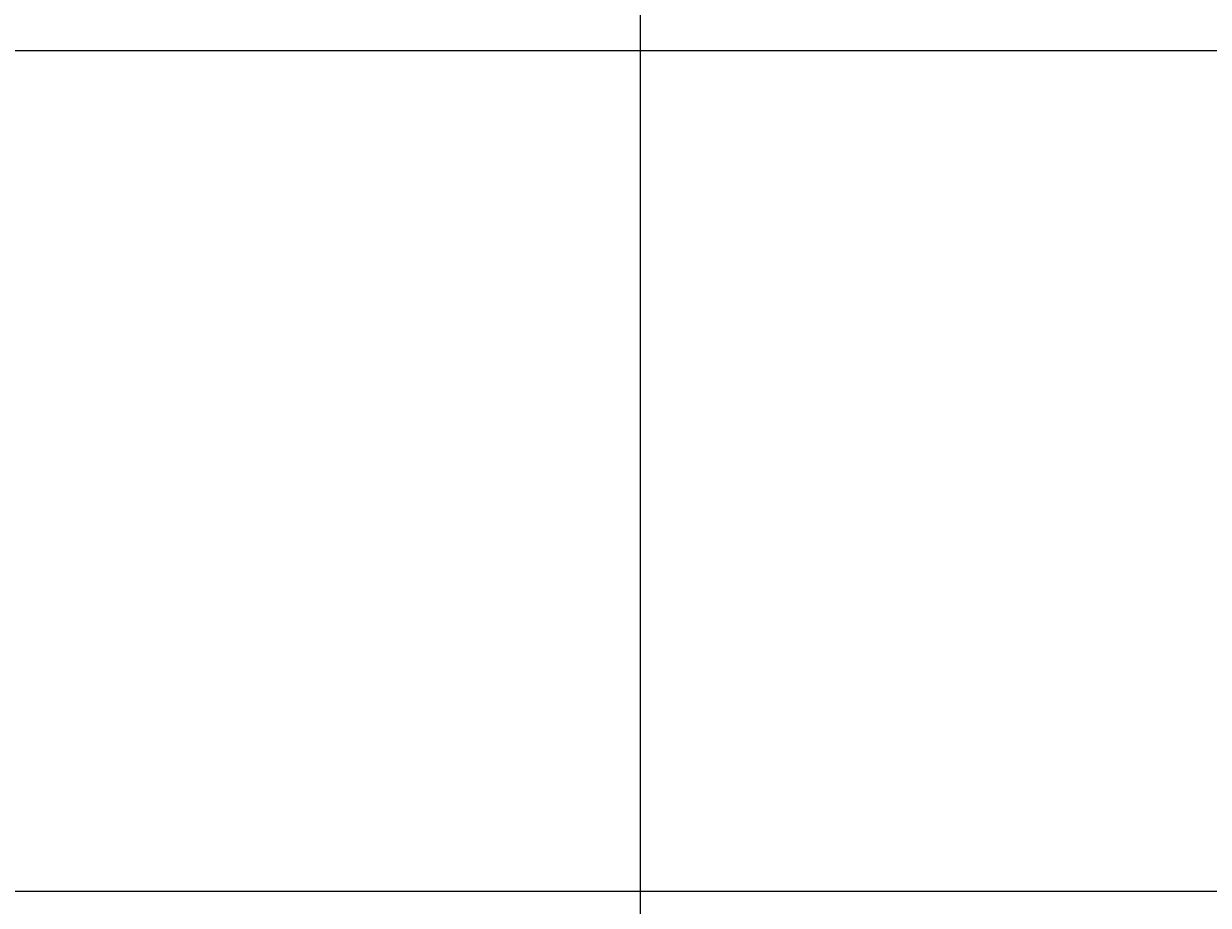
# Model space of a CAD drawing. Units: inches. Extents: x 35362 to 73946, y 43607 to 67532.
# Tile 92 of 134: x 49711 to 50119, y 48965 to 49269. Entities that reach past the tile are written whole.
import ezdxf

# ---------------------------------------------------------------- set-up
doc = ezdxf.new("R2010")
doc.units = ezdxf.units.IN
doc.header["$MEASUREMENT"] = 0
doc.layers.add('A-ANNO-DIMS', color=2, linetype='Continuous', lineweight=18)
doc.styles.get("Standard").update_dxf_attribs({"font": 'arial.ttf'})
doc.dimstyles.get("Standard").update_dxf_attribs({"dimtxt": 0.18, "dimasz": 0.18, "dimexe": 0.18, "dimexo": 0.0625, "dimgap": 0.09, "dimtad": 0, "dimtih": 1, "dimtoh": 1, "dimdec": 4, "dimzin": 0, "dimdsep": 46, "dimtxsty": 'Standard', "dimcen": 0.09, "dimadec": 0, "dimazin": 0, "dimtfac": 1, "dimtdec": 4, "dimtofl": 0, "dimtmove": 0, "dimatfit": 3, "dimfxl": 1, "dimtolj": 1, "dimtzin": 0, "dimarcsym": 0})

# ---------------------------------------------------------------- blocks, each defined once
blk = doc.blocks.new('*D11')
at = {"layer": 'A-ANNO-DIMS', "color": 0, "lineweight": -2, "transparency": 16777216}
for p, q in [((47978.66, 56028.77), (47978.66, 43606.68)), ((53109.76, 56028.77), (53109.76, 43606.68)), ((47978.84, 43606.86), (50543.87, 43606.86)), ((53109.58, 43606.86), (50544.55, 43606.86))]:
    blk.add_line(p, q, dxfattribs=at)
at = {"layer": 'A-ANNO-DIMS', "color": 0, "transparency": 16777216}
for points in [[(47978.84, 43606.89), (47978.84, 43606.83), (47978.66, 43606.86)], [(53109.58, 43606.89), (53109.58, 43606.83), (53109.76, 43606.86)]]:
    blk.add_solid(points, dxfattribs=at)
at = {"layer": 'Defpoints', "color": 0, "transparency": 16777216}
for p in [(47978.66, 56028.84), (53109.76, 56028.84), (53109.76, 43606.86)]:
    blk.add_point(p, dxfattribs=at)
at = {"layer": 'A-ANNO-DIMS', "color": 0, "transparency": 16777216, "insert": (50544.21, 43606.86), "char_height": 0.18, "attachment_point": 5}
blk.add_mtext('\\A1;5131', dxfattribs=at)
blk = doc.blocks.new('*D13')
at = {"layer": 'A-ANNO-DIMS', "color": 0, "lineweight": -2, "transparency": 16777216}
for p, q in [((48373.49, 51694.02), (48373.49, 43606.68)), ((51029.04, 51694.02), (51029.04, 43606.68)), ((48373.67, 43606.86), (49700.8, 43606.86)), ((51028.86, 43606.86), (49701.73, 43606.86))]:
    blk.add_line(p, q, dxfattribs=at)
at = {"layer": 'A-ANNO-DIMS', "color": 0, "transparency": 16777216}
for points in [[(48373.67, 43606.89), (48373.67, 43606.83), (48373.49, 43606.86)], [(51028.86, 43606.89), (51028.86, 43606.83), (51029.04, 43606.86)]]:
    blk.add_solid(points, dxfattribs=at)
at = {"layer": 'Defpoints', "color": 0, "transparency": 16777216}
for p in [(48373.49, 51694.09), (51029.04, 51694.09), (51029.04, 43606.86)]:
    blk.add_point(p, dxfattribs=at)
at = {"layer": 'A-ANNO-DIMS', "color": 0, "transparency": 16777216, "insert": (49701.27, 43606.86), "char_height": 0.18, "attachment_point": 5}
blk.add_mtext('\\A1;2655.6', dxfattribs=at)
blk = doc.blocks.new('*D17')
at = {"layer": 'A-ANNO-DIMS', "color": 0, "lineweight": -2, "transparency": 16777216}
for p, q in [((49923.31, 61293.22), (49923.31, 43606.68)), ((51913.93, 61293.22), (51913.93, 43606.68)), ((49923.49, 43606.86), (50918.16, 43606.86)), ((51913.75, 43606.86), (50919.07, 43606.86))]:
    blk.add_line(p, q, dxfattribs=at)
at = {"layer": 'A-ANNO-DIMS', "color": 0, "transparency": 16777216}
for points in [[(49923.49, 43606.89), (49923.49, 43606.83), (49923.31, 43606.86)], [(51913.75, 43606.89), (51913.75, 43606.83), (51913.93, 43606.86)]]:
    blk.add_solid(points, dxfattribs=at)
at = {"layer": 'Defpoints', "color": 0, "transparency": 16777216}
for p in [(49923.31, 61293.29), (51913.93, 61293.29), (51913.93, 43606.86)]:
    blk.add_point(p, dxfattribs=at)
at = {"layer": 'A-ANNO-DIMS', "color": 0, "transparency": 16777216, "insert": (50918.62, 43606.86), "char_height": 0.18, "attachment_point": 5}
blk.add_mtext('\\A1;1990.6', dxfattribs=at)
blk = doc.blocks.new('*D67')
at = {"layer": 'A-ANNO-DIMS', "color": 0, "lineweight": -2, "transparency": 16777216}
for p, q in [((56873.54, 53351.53), (35361.77, 53351.53)), ((35361.95, 53351.35), (35361.95, 49400.89)), ((35361.95, 45450.07), (35361.95, 49400.53)), ((53793.58, 45449.89), (35361.77, 45449.89))]:
    blk.add_line(p, q, dxfattribs=at)
at = {"layer": 'A-ANNO-DIMS', "color": 0, "transparency": 16777216}
for points in [[(35361.92, 53351.35), (35361.98, 53351.35), (35361.95, 53351.53)], [(35361.92, 45450.07), (35361.98, 45450.07), (35361.95, 45449.89)]]:
    blk.add_solid(points, dxfattribs=at)
at = {"layer": 'Defpoints', "color": 0, "transparency": 16777216}
for p in [(35361.95, 53351.53), (56873.6, 53351.53), (53793.64, 45449.89)]:
    blk.add_point(p, dxfattribs=at)
at = {"layer": 'A-ANNO-DIMS', "color": 0, "transparency": 16777216, "insert": (35361.95, 49400.71), "char_height": 0.18, "attachment_point": 5}
blk.add_mtext('\\A1;7901.6', dxfattribs=at)
blk = doc.blocks.new('*D84')
at = {"layer": 'A-ANNO-DIMS', "color": 0, "lineweight": -2, "transparency": 16777216}
for p, q in [((55540.23, 49259.94), (35361.77, 49259.94)), ((35361.95, 49259.76), (35361.95, 49115.14)), ((35361.95, 48970.16), (35361.95, 49114.78)), ((55540.23, 48969.98), (35361.77, 48969.98))]:
    blk.add_line(p, q, dxfattribs=at)
at = {"layer": 'A-ANNO-DIMS', "color": 0, "transparency": 16777216}
for points in [[(35361.92, 49259.76), (35361.98, 49259.76), (35361.95, 49259.94)], [(35361.92, 48970.16), (35361.98, 48970.16), (35361.95, 48969.98)]]:
    blk.add_solid(points, dxfattribs=at)
at = {"layer": 'Defpoints', "color": 0, "transparency": 16777216}
for p in [(35361.95, 49259.94), (55540.3, 49259.94), (55540.3, 48969.98)]:
    blk.add_point(p, dxfattribs=at)
at = {"layer": 'A-ANNO-DIMS', "color": 0, "transparency": 16777216, "insert": (35361.95, 49114.96), "char_height": 0.18, "attachment_point": 5}
blk.add_mtext('\\A1;289.96', dxfattribs=at)
blk = doc.blocks.new('*D86')
at = {"layer": 'A-ANNO-DIMS', "color": 0, "lineweight": -2, "transparency": 16777216}
for p, q in [((51285.53, 49320.08), (35361.77, 49320.08)), ((35361.95, 49319.9), (35361.95, 49120.26)), ((35361.95, 48920.26), (35361.95, 49119.9)), ((51285.53, 48920.08), (35361.77, 48920.08))]:
    blk.add_line(p, q, dxfattribs=at)
at = {"layer": 'A-ANNO-DIMS', "color": 0, "transparency": 16777216}
for points in [[(35361.92, 49319.9), (35361.98, 49319.9), (35361.95, 49320.08)], [(35361.92, 48920.26), (35361.98, 48920.26), (35361.95, 48920.08)]]:
    blk.add_solid(points, dxfattribs=at)
at = {"layer": 'Defpoints', "color": 0, "transparency": 16777216}
for p in [(35361.95, 49320.08), (51285.59, 49320.08), (51285.59, 48920.08)]:
    blk.add_point(p, dxfattribs=at)
at = {"layer": 'A-ANNO-DIMS', "color": 0, "transparency": 16777216, "insert": (35361.95, 49120.08), "char_height": 0.18, "attachment_point": 5}
blk.add_mtext('\\A1;400.0', dxfattribs=at)

msp = doc.modelspace()

# ---------------------------------------------------------------- dimensions: what is measured, and where the dimension line sits
at = {"layer": 'A-ANNO-DIMS'}
for base, p1, p2, override, picture, middle in [((51913.931, 43606.859), (49923.307, 61293.286), (51913.931, 61293.286), {"dimdec": 1, "dimlfac": 1, "dimrnd": 0, "dimzin": 0, "dimdsep": 46, "dimlunit": 2}, '*D17', (50918.619, 43606.859)), ((53109.76, 43606.859), (47978.665, 56028.836), (53109.76, 56028.836), {"dimdec": 0, "dimlfac": 1, "dimrnd": 0, "dimzin": 0, "dimdsep": 46, "dimlunit": 2}, '*D11', (50544.212, 43606.859)), ((51029.043, 43606.859), (48373.492, 51694.087), (51029.043, 51694.087), {"dimdec": 1, "dimlfac": 1, "dimrnd": 0, "dimzin": 0, "dimdsep": 46, "dimlunit": 2}, '*D13', (49701.267, 43606.859))]:
    dim = msp.add_linear_dim(base=base, p1=p1, p2=p2, dimstyle='Standard', override=override, dxfattribs=at)
    dim.commit()
    dim.dimension.update_dxf_attribs({"geometry": picture, "text_midpoint": middle})
for base, p1, p2, override, picture, middle in [((35361.949, 53351.529), (53793.638, 45449.894), (56873.602, 53351.529), {"dimdec": 1, "dimlfac": 1, "dimrnd": 0, "dimzin": 0, "dimdsep": 46, "dimlunit": 2}, '*D67', (35361.949, 49400.712)), ((35361.949, 49320.079), (51285.595, 48920.079), (51285.595, 49320.079), {"dimdec": 1, "dimlfac": 1, "dimrnd": 0, "dimzin": 0, "dimdsep": 46, "dimlunit": 2}, '*D86', (35361.949, 49120.079)), ((35361.9491, 49259.9353), (55540.2972, 48969.9796), (55540.2972, 49259.9353), {"dimdec": 2, "dimlfac": 1, "dimrnd": 0, "dimzin": 0, "dimdsep": 46, "dimlunit": 2}, '*D84', (35361.9491, 49114.9575))]:
    dim = msp.add_linear_dim(base=base, p1=p1, p2=p2, angle=90, dimstyle='Standard', override=override, dxfattribs=at)
    dim.commit()
    dim.dimension.update_dxf_attribs({"geometry": picture, "text_midpoint": middle})

doc.saveas('drawing.dxf')
